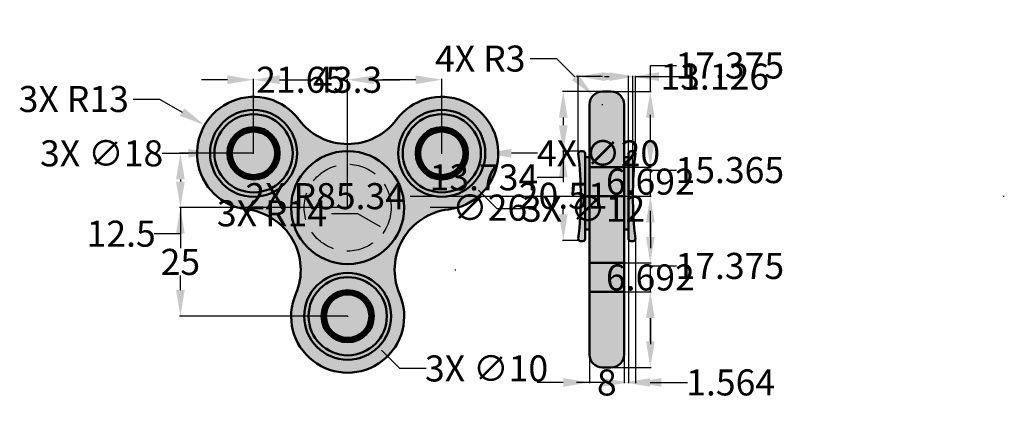
# Model space of a CAD drawing. Units: millimetres. Extents: x 23 to 250, y -22 to 67.
import ezdxf

# ---------------------------------------------------------------- set-up
doc = ezdxf.new("R2010")
doc.units = ezdxf.units.MM
doc.header["$MEASUREMENT"] = 0
doc.linetypes.add('HIDDEN', pattern=[9.525, 6.35, -3.175])
for name, color, linetype, lineweight in [('M-DIMS', 2, 'Continuous', 18), ('M-HATC', 8, 'Continuous', 18), ('M-HIDN', 4, 'HIDDEN', 25), ('M-OUTL', 7, 'Continuous', 50)]:
    doc.layers.add(name, color=color, linetype=linetype, lineweight=lineweight)
doc.styles.get("Standard").update_dxf_attribs({"font": 'arial.ttf'})
doc.dimstyles.get("Standard").update_dxf_attribs({"dimtxt": 6, "dimasz": 6, "dimexe": 0.18, "dimexo": 0.0625, "dimgap": 0.09, "dimtad": 0, "dimtih": 1, "dimtoh": 1, "dimdec": 1, "dimzin": 0, "dimdsep": 46, "dimtxsty": 'Standard', "dimcen": 0.09, "dimadec": 0, "dimazin": 0, "dimtfac": 1, "dimtdec": 1, "dimtofl": 0, "dimtmove": 0, "dimatfit": 3, "dimfxl": 1, "dimtolj": 1, "dimtzin": 0, "dimarcsym": 0})

# ---------------------------------------------------------------- blocks, each defined once
blk = doc.blocks.new('BEARING-SEAT')
for radius in [10, 9, 6, 5]:
    blk.add_circle((10, 10), radius)
blk = doc.blocks.new('FINGER-CAP')
for p, q in [((0.5, 20.69), (1.07, 20.69)), ((0, 10.34), (0, 20.19)), ((0, 10.34), (0, 0.5)), ((0.5, 0), (1.07, 0))]:
    blk.add_line(p, q)
for centre, radius, start, end in [((0.5, 20.19), 0.5, 90, 180), ((1.07, 20.19), 0.5, 353.4148, 90), ((86.34, 10.34), 85.34, 173.4148, 186.5852), ((0.5, 0.5), 0.5, 180, 270), ((1.07, 0.5), 0.5, 270, 6.5852)]:
    blk.add_arc(centre, radius, start, end)
blk = doc.blocks.new('*D3')
at = {"layer": 'Defpoints', "color": 0, "lineweight": 30, "transparency": 16777216}
for p in [(120.56, 53.06), (77.26, 36.13), (120.56, 36.13)]:
    blk.add_point(p, dxfattribs=at)
at = {"layer": 'M-DIMS', "color": 0, "lineweight": -2, "transparency": 16777216}
for p, q in [((77.26, 36.19), (77.26, 53.24)), ((83.26, 53.06), (90.91, 53.06)), ((114.56, 53.06), (106.92, 53.06)), ((120.56, 36.19), (120.56, 53.24))]:
    blk.add_line(p, q, dxfattribs=at)
at = {"layer": 'M-DIMS', "color": 0, "lineweight": 30, "transparency": 16777216}
for points in [[(83.26, 54.06), (83.26, 52.06), (77.26, 53.06)], [(114.56, 54.06), (114.56, 52.06), (120.56, 53.06)]]:
    blk.add_solid(points, dxfattribs=at)
at = {"layer": 'M-DIMS', "color": 0, "transparency": 16777216, "insert": (98.91, 53.06), "char_height": 6, "attachment_point": 5}
blk.add_mtext('\\A1;43.3', dxfattribs=at)
blk = doc.blocks.new('*D4')
at = {"layer": 'Defpoints', "color": 0, "lineweight": 30, "transparency": 16777216}
for p in [(98.91, 53.06), (77.26, 36.13), (98.91, 23.63)]:
    blk.add_point(p, dxfattribs=at)
at = {"layer": 'M-DIMS', "color": 0, "lineweight": -2, "transparency": 16777216}
for p, q in [((71.26, 53.06), (65.26, 53.06)), ((77.26, 36.19), (77.26, 53.24)), ((98.91, 23.69), (98.91, 53.24)), ((104.91, 53.06), (110.91, 53.06))]:
    blk.add_line(p, q, dxfattribs=at)
at = {"layer": 'M-DIMS', "color": 0, "lineweight": 30, "transparency": 16777216}
for points in [[(71.26, 54.06), (71.26, 52.06), (77.26, 53.06)], [(104.91, 54.06), (104.91, 52.06), (98.91, 53.06)]]:
    blk.add_solid(points, dxfattribs=at)
at = {"layer": 'M-DIMS', "color": 0, "transparency": 16777216, "insert": (88.09, 53.06), "char_height": 6, "attachment_point": 5}
blk.add_mtext('\\A1;21.65', dxfattribs=at)
blk = doc.blocks.new('*D5')
at = {"layer": 'Defpoints', "color": 0, "lineweight": 30, "transparency": 16777216}
for p in [(77.26, 36.13), (60.43, 23.63), (98.91, 23.63)]:
    blk.add_point(p, dxfattribs=at)
at = {"layer": 'M-DIMS', "color": 0, "lineweight": -2, "transparency": 16777216}
for p, q in [((77.2, 36.13), (60.25, 36.13)), ((60.43, 30.13), (60.43, 29.63)), ((98.85, 23.63), (60.25, 23.63)), ((60.43, 23.63), (60.43, 17.63)), ((60.43, 17.63), (54.43, 17.63))]:
    blk.add_line(p, q, dxfattribs=at)
at = {"layer": 'M-DIMS', "color": 0, "lineweight": 30, "transparency": 16777216}
for points in [[(59.43, 30.13), (61.43, 30.13), (60.43, 36.13)], [(59.43, 29.63), (61.43, 29.63), (60.43, 23.63)]]:
    blk.add_solid(points, dxfattribs=at)
at = {"layer": 'M-DIMS', "color": 0, "transparency": 16777216, "insert": (46.81, 17.63), "char_height": 6, "attachment_point": 5}
blk.add_mtext('\\A1;12.5', dxfattribs=at)
blk = doc.blocks.new('*D6')
at = {"layer": 'Defpoints', "color": 0, "lineweight": 30, "transparency": 16777216}
for p in [(98.91, 23.63), (60.43, -1.37), (98.91, -1.37)]:
    blk.add_point(p, dxfattribs=at)
at = {"layer": 'M-DIMS', "color": 0, "lineweight": -2, "transparency": 16777216}
for p, q in [((98.85, 23.63), (60.25, 23.63)), ((60.43, 17.63), (60.43, 14.28)), ((60.43, 4.63), (60.43, 7.97)), ((98.85, -1.37), (60.25, -1.37))]:
    blk.add_line(p, q, dxfattribs=at)
at = {"layer": 'M-DIMS', "color": 0, "lineweight": 30, "transparency": 16777216}
for points in [[(59.43, 17.63), (61.43, 17.63), (60.43, 23.63)], [(59.43, 4.63), (61.43, 4.63), (60.43, -1.37)]]:
    blk.add_solid(points, dxfattribs=at)
at = {"layer": 'M-DIMS', "color": 0, "transparency": 16777216, "insert": (60.43, 11.13), "char_height": 6, "attachment_point": 5}
blk.add_mtext('\\A1;25', dxfattribs=at)
blk = doc.blocks.new('*D7')
at = {"layer": 'Defpoints', "color": 0, "lineweight": 30, "transparency": 16777216}
for p in [(154.514575, -10.163581), (162.514575, -10.163581), (162.514575, -16.613581)]:
    blk.add_point(p, dxfattribs=at)
at = {"layer": 'M-DIMS', "color": 0, "lineweight": -2, "transparency": 16777216}
for p, q in [((154.514575, -10.226081), (154.514575, -16.793581)), ((162.514575, -10.226081), (162.514575, -16.793581)), ((148.514575, -16.613581), (142.514575, -16.613581)), ((168.514575, -16.613581), (174.514575, -16.613581))]:
    blk.add_line(p, q, dxfattribs=at)
at = {"layer": 'M-DIMS', "color": 0, "lineweight": 30, "transparency": 16777216}
for points in [[(148.514575, -15.613581), (148.514575, -17.613581), (154.514575, -16.613581)], [(168.514575, -15.613581), (168.514575, -17.613581), (162.514575, -16.613581)]]:
    blk.add_solid(points, dxfattribs=at)
at = {"layer": 'M-DIMS', "color": 0, "transparency": 16777216, "insert": (158.514575, -16.613581), "char_height": 6, "attachment_point": 5}
blk.add_mtext('\\A1;8', dxfattribs=at)
blk = doc.blocks.new('*D8')
at = {"layer": 'Defpoints', "color": 0, "lineweight": 30, "transparency": 16777216}
for p in [(165.08, 53.79), (151.95, 36.06), (165.08, 36.06)]:
    blk.add_point(p, dxfattribs=at)
at = {"layer": 'M-DIMS', "color": 0, "lineweight": -2, "transparency": 16777216}
for p, q in [((151.95, 36.12), (151.95, 53.97)), ((157.95, 53.79), (159.08, 53.79)), ((165.08, 36.12), (165.08, 53.97)), ((165.08, 53.79), (171.08, 53.79))]:
    blk.add_line(p, q, dxfattribs=at)
at = {"layer": 'M-DIMS', "color": 0, "lineweight": 30, "transparency": 16777216}
for points in [[(157.95, 54.79), (157.95, 52.79), (151.95, 53.79)], [(159.08, 54.79), (159.08, 52.79), (165.08, 53.79)]]:
    blk.add_solid(points, dxfattribs=at)
at = {"layer": 'M-DIMS', "color": 0, "transparency": 16777216, "insert": (183.34, 53.79), "char_height": 6, "attachment_point": 5}
blk.add_mtext('\\A1;13.126', dxfattribs=at)
blk = doc.blocks.new('*D9')
at = {"layer": 'Defpoints', "color": 0, "lineweight": 30, "transparency": 16777216}
for p in [(157.51, 50.34), (148.5, 36.6), (152.34, 36.6)]:
    blk.add_point(p, dxfattribs=at)
at = {"layer": 'M-DIMS', "color": 0, "lineweight": -2, "transparency": 16777216}
for p, q in [((157.45, 50.34), (148.32, 50.34)), ((148.5, 44.34), (148.5, 42.6)), ((152.28, 36.6), (148.32, 36.6)), ((148.5, 36.6), (148.5, 30.6)), ((148.5, 30.6), (142.5, 30.6))]:
    blk.add_line(p, q, dxfattribs=at)
at = {"layer": 'M-DIMS', "color": 0, "lineweight": 30, "transparency": 16777216}
for points in [[(147.5, 44.34), (149.5, 44.34), (148.5, 50.34)], [(147.5, 42.6), (149.5, 42.6), (148.5, 36.6)]]:
    blk.add_solid(points, dxfattribs=at)
at = {"layer": 'M-DIMS', "color": 0, "transparency": 16777216, "insert": (130.25, 30.6), "char_height": 6, "attachment_point": 5}
blk.add_mtext('\\A1;13.734', dxfattribs=at)
blk = doc.blocks.new('*D10')
at = {"layer": 'Defpoints', "color": 0, "lineweight": 30, "transparency": 16777216}
for p in [(152.34, 36.6), (148.5, 16.09), (152.07, 16.09)]:
    blk.add_point(p, dxfattribs=at)
at = {"layer": 'M-DIMS', "color": 0, "lineweight": -2, "transparency": 16777216}
for p, q in [((152.28, 36.6), (148.32, 36.6)), ((148.5, 30.6), (148.5, 29.5)), ((148.5, 22.09), (148.5, 23.19)), ((152.01, 16.09), (148.32, 16.09))]:
    blk.add_line(p, q, dxfattribs=at)
at = {"layer": 'M-DIMS', "color": 0, "lineweight": 30, "transparency": 16777216}
for points in [[(147.5, 30.6), (149.5, 30.6), (148.5, 36.6)], [(147.5, 22.09), (149.5, 22.09), (148.5, 16.09)]]:
    blk.add_solid(points, dxfattribs=at)
at = {"layer": 'M-DIMS', "color": 0, "transparency": 16777216, "insert": (148.5, 26.35), "char_height": 6, "attachment_point": 5}
blk.add_mtext('\\A1;20.51', dxfattribs=at)
blk = doc.blocks.new('*D11')
at = {"layer": 'Defpoints', "color": 0, "lineweight": 30, "transparency": 16777216}
for p in [(162.51, 4.21), (168.53, 4.21), (159.51, -13.16)]:
    blk.add_point(p, dxfattribs=at)
at = {"layer": 'M-DIMS', "color": 0, "lineweight": -2, "transparency": 16777216}
for p, q in [((168.53, 4.21), (168.53, 10.21)), ((168.53, 10.21), (174.53, 10.21)), ((162.58, 4.21), (168.71, 4.21)), ((168.53, -7.16), (168.53, -1.79)), ((159.58, -13.16), (168.71, -13.16))]:
    blk.add_line(p, q, dxfattribs=at)
at = {"layer": 'M-DIMS', "color": 0, "lineweight": 30, "transparency": 16777216}
for points in [[(167.53, -1.79), (169.53, -1.79), (168.53, 4.21)], [(167.53, -7.16), (169.53, -7.16), (168.53, -13.16)]]:
    blk.add_solid(points, dxfattribs=at)
at = {"layer": 'M-DIMS', "color": 0, "transparency": 16777216, "insert": (186.81, 10.21), "char_height": 6, "attachment_point": 5}
blk.add_mtext('\\A1;17.375', dxfattribs=at)
blk = doc.blocks.new('*D12')
at = {"layer": 'Defpoints', "color": 0, "lineweight": 30, "transparency": 16777216}
for p in [(162.514575, 10.903671), (168.528589, 10.903671), (162.514575, 4.211419)]:
    blk.add_point(p, dxfattribs=at)
at = {"layer": 'M-DIMS', "color": 0, "lineweight": -2, "transparency": 16777216}
for p, q in [((168.528589, 16.903671), (168.528589, 22.903671)), ((162.577075, 10.903671), (168.708589, 10.903671)), ((162.577075, 4.211419), (168.708589, 4.211419)), ((168.528589, -1.788581), (168.528589, -7.788581))]:
    blk.add_line(p, q, dxfattribs=at)
at = {"layer": 'M-DIMS', "color": 0, "lineweight": 30, "transparency": 16777216}
for points in [[(167.528589, 16.903671), (169.528589, 16.903671), (168.528589, 10.903671)], [(167.528589, -1.788581), (169.528589, -1.788581), (168.528589, 4.211419)]]:
    blk.add_solid(points, dxfattribs=at)
at = {"layer": 'M-DIMS', "color": 0, "transparency": 16777216, "insert": (168.528589, 7.557545), "char_height": 6, "attachment_point": 5}
blk.add_mtext('\\A1;6.692', dxfattribs=at)
blk = doc.blocks.new('*D13')
at = {"layer": 'Defpoints', "color": 0, "lineweight": 30, "transparency": 16777216}
for p in [(162.51, 26.27), (168.53, 26.27), (162.51, 10.9)]:
    blk.add_point(p, dxfattribs=at)
at = {"layer": 'M-DIMS', "color": 0, "lineweight": -2, "transparency": 16777216}
for p, q in [((168.53, 26.27), (168.53, 32.27)), ((168.53, 32.27), (174.53, 32.27)), ((162.58, 26.27), (168.71, 26.27)), ((168.53, 16.9), (168.53, 20.27)), ((162.58, 10.9), (168.71, 10.9))]:
    blk.add_line(p, q, dxfattribs=at)
at = {"layer": 'M-DIMS', "color": 0, "lineweight": 30, "transparency": 16777216}
for points in [[(167.53, 20.27), (169.53, 20.27), (168.53, 26.27)], [(167.53, 16.9), (169.53, 16.9), (168.53, 10.9)]]:
    blk.add_solid(points, dxfattribs=at)
at = {"layer": 'M-DIMS', "color": 0, "transparency": 16777216, "insert": (186.81, 32.27), "char_height": 6, "attachment_point": 5}
blk.add_mtext('\\A1;15.365', dxfattribs=at)
blk = doc.blocks.new('*D14')
at = {"layer": 'Defpoints', "color": 0, "lineweight": 30, "transparency": 16777216}
for p in [(162.514575, 32.961419), (168.528589, 32.961419), (162.514575, 26.269167)]:
    blk.add_point(p, dxfattribs=at)
at = {"layer": 'M-DIMS', "color": 0, "lineweight": -2, "transparency": 16777216}
for p, q in [((168.528589, 38.961419), (168.528589, 44.961419)), ((162.577075, 32.961419), (168.708589, 32.961419)), ((162.577075, 26.269167), (168.708589, 26.269167)), ((168.528589, 20.269167), (168.528589, 14.269167))]:
    blk.add_line(p, q, dxfattribs=at)
at = {"layer": 'M-DIMS', "color": 0, "lineweight": 30, "transparency": 16777216}
for points in [[(167.528589, 38.961419), (169.528589, 38.961419), (168.528589, 32.961419)], [(167.528589, 20.269167), (169.528589, 20.269167), (168.528589, 26.269167)]]:
    blk.add_solid(points, dxfattribs=at)
at = {"layer": 'M-DIMS', "color": 0, "transparency": 16777216, "insert": (168.528589, 29.615293), "char_height": 6, "attachment_point": 5}
blk.add_mtext('\\A1;6.692', dxfattribs=at)
blk = doc.blocks.new('*D15')
at = {"layer": 'Defpoints', "color": 0, "lineweight": 30, "transparency": 16777216}
for p in [(159.51, 50.34), (168.53, 50.34), (162.51, 32.96)]:
    blk.add_point(p, dxfattribs=at)
at = {"layer": 'M-DIMS', "color": 0, "lineweight": -2, "transparency": 16777216}
for p, q in [((168.53, 50.34), (168.53, 56.34)), ((168.53, 56.34), (174.53, 56.34)), ((159.58, 50.34), (168.71, 50.34)), ((168.53, 38.96), (168.53, 44.34)), ((162.58, 32.96), (168.71, 32.96))]:
    blk.add_line(p, q, dxfattribs=at)
at = {"layer": 'M-DIMS', "color": 0, "lineweight": 30, "transparency": 16777216}
for points in [[(167.53, 44.34), (169.53, 44.34), (168.53, 50.34)], [(167.53, 38.96), (169.53, 38.96), (168.53, 32.96)]]:
    blk.add_solid(points, dxfattribs=at)
at = {"layer": 'M-DIMS', "color": 0, "transparency": 16777216, "insert": (186.81, 56.34), "char_height": 6, "attachment_point": 5}
blk.add_mtext('\\A1;17.375', dxfattribs=at)
blk = doc.blocks.new('*D16')
at = {"layer": 'Defpoints', "color": 0, "lineweight": 30, "transparency": 16777216}
for p in [(163.51, 16.42), (165.08, 16.38), (165.08, -16.61)]:
    blk.add_point(p, dxfattribs=at)
at = {"layer": 'M-DIMS', "color": 0, "lineweight": -2, "transparency": 16777216}
for p, q in [((163.51, 16.36), (163.51, -16.79)), ((165.08, 16.31), (165.08, -16.79)), ((157.51, -16.61), (151.51, -16.61)), ((171.08, -16.61), (177.08, -16.61))]:
    blk.add_line(p, q, dxfattribs=at)
at = {"layer": 'M-DIMS', "color": 0, "lineweight": 30, "transparency": 16777216}
for points in [[(157.51, -15.61), (157.51, -17.61), (163.51, -16.61)], [(171.08, -15.61), (171.08, -17.61), (165.08, -16.61)]]:
    blk.add_solid(points, dxfattribs=at)
at = {"layer": 'M-DIMS', "color": 0, "transparency": 16777216, "insert": (187, -16.61), "char_height": 6, "attachment_point": 5}
blk.add_mtext('\\A1;1.564', dxfattribs=at)
blk = doc.blocks.new('*D17')
at = {"layer": 'Defpoints', "color": 0, "lineweight": 30, "transparency": 16777216}
for p in [(164.51, 53.79), (163.51, 26.27), (164.51, 26.27)]:
    blk.add_point(p, dxfattribs=at)
at = {"layer": 'M-DIMS', "color": 0, "lineweight": -2, "transparency": 16777216}
for p, q in [((157.51, 53.79), (151.51, 53.79)), ((163.51, 26.33), (163.51, 53.97)), ((164.51, 26.33), (164.51, 53.97)), ((170.51, 53.79), (176.51, 53.79))]:
    blk.add_line(p, q, dxfattribs=at)
at = {"layer": 'M-DIMS', "color": 0, "lineweight": 30, "transparency": 16777216}
for points in [[(157.51, 54.79), (157.51, 52.79), (163.51, 53.79)], [(170.51, 54.79), (170.51, 52.79), (164.51, 53.79)]]:
    blk.add_solid(points, dxfattribs=at)
at = {"layer": 'M-DIMS', "color": 0, "transparency": 16777216, "insert": (177.71, 53.79), "char_height": 6, "attachment_point": 5}
blk.add_mtext('\\A1;1', dxfattribs=at)
blk = doc.blocks.new('*D18')
at = {"layer": 'Defpoints', "color": 0, "lineweight": 30, "transparency": 16777216}
for p in [(85.91, 23.63), (111.91, 23.63)]:
    blk.add_point(p, dxfattribs=at)
at = {"layer": 'M-DIMS', "color": 0, "lineweight": -2, "transparency": 16777216}
for p, q in [((98.82, 23.63), (99, 23.63)), ((98.91, 23.54), (98.91, 23.72)), ((123.91, 23.63), (117.91, 23.63))]:
    blk.add_line(p, q, dxfattribs=at)
at = {"layer": 'M-DIMS', "color": 0, "lineweight": 30, "transparency": 16777216}
blk.add_solid([(117.91, 24.63), (117.91, 22.63), (111.91, 23.63)], dxfattribs=at)
at = {"layer": 'M-DIMS', "color": 0, "transparency": 16777216, "insert": (131.56, 23.63), "char_height": 6, "attachment_point": 5}
blk.add_mtext('\\A1;∅26', dxfattribs=at)
blk = doc.blocks.new('*D19')
at = {"layer": 'Defpoints', "color": 0, "lineweight": 30, "transparency": 16777216}
for p in [(110.56, 36.13), (130.56, 36.13)]:
    blk.add_point(p, dxfattribs=at)
at = {"layer": 'M-DIMS', "color": 0, "lineweight": -2, "transparency": 16777216}
for p, q in [((120.47, 36.13), (120.65, 36.13)), ((120.56, 36.04), (120.56, 36.22)), ((142.56, 36.13), (136.56, 36.13))]:
    blk.add_line(p, q, dxfattribs=at)
at = {"layer": 'M-DIMS', "color": 0, "lineweight": 30, "transparency": 16777216}
blk.add_solid([(136.56, 37.13), (136.56, 35.13), (130.56, 36.13)], dxfattribs=at)
at = {"layer": 'M-DIMS', "color": 0, "transparency": 16777216, "insert": (156.61, 36.13), "char_height": 6, "attachment_point": 5}
blk.add_mtext('\\A1;4X ∅20', dxfattribs=at)
blk = doc.blocks.new('*D20')
at = {"layer": 'Defpoints', "color": 0, "lineweight": 30, "transparency": 16777216}
for p in [(68.26, 36.13), (86.26, 36.13)]:
    blk.add_point(p, dxfattribs=at)
at = {"layer": 'M-DIMS', "color": 0, "lineweight": -2, "transparency": 16777216}
for p, q in [((56.26, 36.13), (62.26, 36.13)), ((77.17, 36.13), (77.35, 36.13)), ((77.26, 36.04), (77.26, 36.22))]:
    blk.add_line(p, q, dxfattribs=at)
at = {"layer": 'M-DIMS', "color": 0, "lineweight": 30, "transparency": 16777216}
blk.add_solid([(62.26, 37.13), (62.26, 35.13), (68.26, 36.13)], dxfattribs=at)
at = {"layer": 'M-DIMS', "color": 0, "transparency": 16777216, "insert": (42.32, 36.13), "char_height": 6, "attachment_point": 5}
blk.add_mtext('\\A1;3X ∅18', dxfattribs=at)
blk = doc.blocks.new('*D21')
at = {"layer": 'Defpoints', "color": 0, "lineweight": 30, "transparency": 16777216}
for p in [(116.33, 40.37), (124.8, 31.88)]:
    blk.add_point(p, dxfattribs=at)
at = {"layer": 'M-DIMS', "color": 0, "lineweight": -2, "transparency": 16777216}
for p, q in [((120.47, 36.13), (120.65, 36.13)), ((120.56, 36.04), (120.56, 36.22)), ((133.28, 23.38), (129.04, 27.63)), ((139.28, 23.38), (133.28, 23.38))]:
    blk.add_line(p, q, dxfattribs=at)
at = {"layer": 'M-DIMS', "color": 0, "lineweight": 30, "transparency": 16777216}
blk.add_solid([(129.75, 28.34), (128.33, 26.93), (124.8, 31.88)], dxfattribs=at)
at = {"layer": 'M-DIMS', "color": 0, "transparency": 16777216, "insert": (153.18, 23.38), "char_height": 6, "attachment_point": 5}
blk.add_mtext('\\A1;3X ∅12', dxfattribs=at)
blk = doc.blocks.new('*D22')
at = {"layer": 'Defpoints', "color": 0, "lineweight": 30, "transparency": 16777216}
for p in [(95.38, 2.16), (102.45, -4.91)]:
    blk.add_point(p, dxfattribs=at)
at = {"layer": 'M-DIMS', "color": 0, "lineweight": -2, "transparency": 16777216}
for p, q in [((98.82, -1.37), (99, -1.37)), ((98.91, -1.46), (98.91, -1.28)), ((110.93, -13.39), (106.69, -9.15)), ((116.93, -13.39), (110.93, -13.39))]:
    blk.add_line(p, q, dxfattribs=at)
at = {"layer": 'M-DIMS', "color": 0, "lineweight": 30, "transparency": 16777216}
blk.add_solid([(107.4, -8.44), (105.98, -9.86), (102.45, -4.91)], dxfattribs=at)
at = {"layer": 'M-DIMS', "color": 0, "transparency": 16777216, "insert": (130.86, -13.39), "char_height": 6, "attachment_point": 5}
blk.add_mtext('\\A1;3X ∅10', dxfattribs=at)
blk = doc.blocks.new('*D23')
at = {"layer": 'Defpoints', "color": 0, "lineweight": 30, "transparency": 16777216}
for p in [(66, 42.63), (77.26, 36.13)]:
    blk.add_point(p, dxfattribs=at)
at = {"layer": 'M-DIMS', "color": 0, "lineweight": -2, "transparency": 16777216}
for p, q in [((49.61, 48.63), (55.61, 48.63)), ((55.61, 48.63), (60.81, 45.63)), ((77.17, 36.13), (77.35, 36.13)), ((77.26, 36.04), (77.26, 36.22))]:
    blk.add_line(p, q, dxfattribs=at)
at = {"layer": 'M-DIMS', "color": 0, "lineweight": 30, "transparency": 16777216}
blk.add_solid([(61.31, 46.49), (60.31, 44.76), (66, 42.63)], dxfattribs=at)
at = {"layer": 'M-DIMS', "color": 0, "transparency": 16777216, "insert": (35.91, 48.63), "char_height": 6, "attachment_point": 5}
blk.add_mtext('\\A1;3X R13', dxfattribs=at)
blk = doc.blocks.new('*D24')
at = {"layer": 'Defpoints', "color": 0, "lineweight": 30, "transparency": 16777216}
for p in [(111.58, 16.31), (123.71, 9.31)]:
    blk.add_point(p, dxfattribs=at)
at = {"layer": 'M-DIMS', "color": 0, "lineweight": -2, "transparency": 16777216}
for p, q in [((95.19, 22.31), (101.19, 22.31)), ((101.19, 22.31), (106.39, 19.31)), ((123.62, 9.31), (123.8, 9.31)), ((123.71, 9.22), (123.71, 9.4))]:
    blk.add_line(p, q, dxfattribs=at)
at = {"layer": 'M-DIMS', "color": 0, "lineweight": 30, "transparency": 16777216}
blk.add_solid([(106.89, 20.18), (105.89, 18.45), (111.58, 16.31)], dxfattribs=at)
at = {"layer": 'M-DIMS', "color": 0, "transparency": 16777216, "insert": (81.5, 22.31), "char_height": 6, "attachment_point": 5}
blk.add_mtext('\\A1;3X R14', dxfattribs=at)
blk = doc.blocks.new('*D25')
at = {"layer": 'Defpoints', "color": 0, "lineweight": 30, "transparency": 16777216}
for p in [(164.51, 26.27), (249.86, 26.27)]:
    blk.add_point(p, dxfattribs=at)
at = {"layer": 'M-DIMS', "color": 0, "lineweight": -2, "transparency": 16777216}
for p, q in [((113.31, 26.27), (158.51, 26.27)), ((249.77, 26.27), (249.95, 26.27)), ((249.86, 26.18), (249.86, 26.36))]:
    blk.add_line(p, q, dxfattribs=at)
at = {"layer": 'M-DIMS', "color": 0, "lineweight": 30, "transparency": 16777216}
blk.add_solid([(158.51, 27.27), (158.51, 25.27), (164.51, 26.27)], dxfattribs=at)
at = {"layer": 'M-DIMS', "color": 0, "transparency": 16777216, "insert": (93.74, 26.27), "char_height": 6, "attachment_point": 5}
blk.add_mtext('\\A1;2X R85.34', dxfattribs=at)
blk = doc.blocks.new('*D26')
at = {"layer": 'Defpoints', "color": 0, "lineweight": 30, "transparency": 16777216}
for p in [(155.39, 49.46), (157.51, 47.34)]:
    blk.add_point(p, dxfattribs=at)
at = {"layer": 'M-DIMS', "color": 0, "lineweight": -2, "transparency": 16777216}
for p, q in [((140.91, 57.94), (146.91, 57.94)), ((146.91, 57.94), (151.15, 53.7)), ((157.42, 47.34), (157.6, 47.34)), ((157.51, 47.25), (157.51, 47.43))]:
    blk.add_line(p, q, dxfattribs=at)
at = {"layer": 'M-DIMS', "color": 0, "lineweight": 30, "transparency": 16777216}
blk.add_solid([(151.86, 54.41), (150.44, 52.99), (155.39, 49.46)], dxfattribs=at)
at = {"layer": 'M-DIMS', "color": 0, "transparency": 16777216, "insert": (129.41, 57.94), "char_height": 6, "attachment_point": 5}
blk.add_mtext('\\A1;4X R3', dxfattribs=at)

msp = doc.modelspace()

# ---------------------------------------------------------------- hatches: boundary and pattern name
at = {"layer": 'M-HATC'}
h = msp.add_hatch(color=256, dxfattribs=at)
h.dxf.hatch_style = 1
h.set_gradient(color1=(237, 31, 36), color2=(248, 153, 30), tint=1)
h.paths.add_polyline_path([(162.5146, 47.3364, 0.41421356), (159.5146, 50.3364), (157.5146, 50.3364, 0.41421356), (154.5146, 47.3364), (154.5146, 32.9614), (162.5146, 32.9614), (162.5146, 35.2241)])
h.paths.add_polyline_path([(162.5146, 26.2692), (154.5146, 26.2692), (154.5146, 10.9037), (162.5146, 10.9037)])
h.paths.add_polyline_path([(162.5146, 4.2114), (154.5146, 4.2114), (154.5146, -10.1636, 0.41421356), (157.5146, -13.1636), (159.5146, -13.1636, 0.41421356), (162.5146, -10.1636)])
h = msp.add_hatch(color=256, dxfattribs=at)
h.dxf.hatch_style = 1
h.set_gradient(color1=(205, 32, 39), color2=(255, 255, 0), tint=1)
h.paths.add_polyline_path([(110.139, 43.8941, -0.50195914), (87.6865, 43.8941, 1.51973937), (75.7475, 23.2152, -0.50195914), (86.9738, 3.7708, 1.51973937), (110.8517, 3.7708, -0.50195914), (122.0779, 23.2152, 1.51973937)])
h.paths.add_polyline_path([(111.9127, 23.6267, -1), (85.9127, 23.6267, -1)], flags=16)
h.paths.add_polyline_path([(67.2621, 36.1267, -1), (87.2621, 36.1267, -1)], flags=16)
h.paths.add_polyline_path([(108.9127, 23.6267, -1), (88.9127, 23.6267, -1)], flags=0)
h.paths.add_polyline_path([(68.2621, 36.1267, -1), (86.2621, 36.1267, -1)], flags=0)
h.paths.add_polyline_path([(71.2621, 36.1267, -1), (83.2621, 36.1267, -1)], flags=0)
h.paths.add_polyline_path([(72.2621, 36.1267, -1), (82.2621, 36.1267, -1)], flags=0)
h.paths.add_polyline_path([(108.9127, -1.3733, -1), (88.9127, -1.3733, -1)], flags=16)
h.paths.add_polyline_path([(107.9127, -1.3733, -1), (89.9127, -1.3733, -1)], flags=0)
h.paths.add_polyline_path([(104.9127, -1.3733, -1), (92.9127, -1.3733, -1)], flags=0)
h.paths.add_polyline_path([(103.9127, -1.3733, -1), (93.9127, -1.3733, -1)], flags=0)
h.paths.add_polyline_path([(110.5633, 36.1267, -1), (130.5633, 36.1267, -1)], flags=16)
h.paths.add_polyline_path([(111.5633, 36.1267, -1), (129.5633, 36.1267, -1)], flags=0)
h.paths.add_polyline_path([(114.5633, 36.1267, -1), (126.5633, 36.1267, -1)], flags=0)
h.paths.add_polyline_path([(115.5633, 36.1267, -1), (125.5633, 36.1267, -1)], flags=0)
h = msp.add_hatch(color=256, dxfattribs=at)
h.dxf.hatch_style = 1
h.set_gradient(color1=(69, 84, 165), color2=(237, 31, 36), tint=1)
h.paths.add_polyline_path([(67.2621, 36.1267, 1), (87.2621, 36.1267, 1)])
h.paths.add_polyline_path([(86.2621, 36.1267, -1), (68.2621, 36.1267, -1)], flags=16)
h.paths.add_polyline_path([(83.2621, 36.1267, -1), (71.2621, 36.1267, -1)], flags=0)
h.paths.add_polyline_path([(82.2621, 36.1267, -1), (72.2621, 36.1267, -1)], flags=0)
h.paths.add_polyline_path([(111.9127, 23.6267, 1), (85.9127, 23.6267, 1)])
h.paths.add_polyline_path([(88.9127, 23.6267, -1), (108.9127, 23.6267, -1)], flags=16)
h.paths.add_polyline_path([(110.5633, 36.1267, 1), (130.5633, 36.1267, 1)])
h.paths.add_polyline_path([(129.5633, 36.1267, -1), (111.5633, 36.1267, -1)], flags=16)
h.paths.add_polyline_path([(126.5633, 36.1267, -1), (114.5633, 36.1267, -1)], flags=0)
h.paths.add_polyline_path([(125.5633, 36.1267, -1), (115.5633, 36.1267, -1)], flags=0)
h.paths.add_polyline_path([(88.9127, -1.3733, 1), (108.9127, -1.3733, 1)])
h.paths.add_polyline_path([(107.9127, -1.3733, -1), (89.9127, -1.3733, -1)], flags=16)
h.paths.add_polyline_path([(104.9127, -1.3733, -1), (92.9127, -1.3733, -1)], flags=0)
h.paths.add_polyline_path([(103.9127, -1.3733, -1), (93.9127, -1.3733, -1)], flags=0)
h = msp.add_hatch(color=256, dxfattribs=at)
h.dxf.hatch_style = 1
h.set_gradient(color1=(205, 32, 39), color2=(255, 255, 0), tint=1)
h.paths.add_polyline_path([(86.2621, 36.1267, 1), (68.2621, 36.1267, 1)])
h.paths.add_polyline_path([(71.2621, 36.1267, -1), (83.2621, 36.1267, -1)], flags=16)
h.paths.add_polyline_path([(72.2621, 36.1267, -1), (82.2621, 36.1267, -1)], flags=0)
h.paths.add_polyline_path([(129.5633, 36.1267, 1), (111.5633, 36.1267, 1)])
h.paths.add_polyline_path([(114.5633, 36.1267, -1), (126.5633, 36.1267, -1)], flags=16)
h.paths.add_polyline_path([(115.5633, 36.1267, -1), (125.5633, 36.1267, -1)], flags=0)
h.paths.add_polyline_path([(89.9127, -1.3733, 1), (107.9127, -1.3733, 1)])
h.paths.add_polyline_path([(104.9127, -1.3733, -1), (92.9127, -1.3733, -1)], flags=16)
h.paths.add_polyline_path([(103.9127, -1.3733, -1), (93.9127, -1.3733, -1)], flags=0)
h = msp.add_hatch(dxfattribs=at)
h.set_pattern_fill('ANSI31', color=256)
h.paths.add_polyline_path([(71.2621, 36.1267, 1), (83.2621, 36.1267, 1)])
h.paths.add_polyline_path([(82.2621, 36.1267, -1), (72.2621, 36.1267, -1)], flags=16)
h.paths.add_polyline_path([(114.5633, 36.1267, 1), (126.5633, 36.1267, 1)])
h.paths.add_polyline_path([(125.5633, 36.1267, -1), (115.5633, 36.1267, -1)], flags=16)
h.paths.add_polyline_path([(104.9127, -1.3733, 1), (92.9127, -1.3733, 1)])
h.paths.add_polyline_path([(93.9127, -1.3733, -1), (103.9127, -1.3733, -1)], flags=16)
h = msp.add_hatch(color=256, dxfattribs=at)
h.dxf.hatch_style = 1
h.set_gradient(color1=(205, 105, 40), color2=(237, 31, 36), tint=1)
h.paths.add_polyline_path([(88.9127, 23.6267, 1), (108.9127, 23.6267, 1)])
h.paths.add_polyline_path([(125.5633, 36.1267, 1), (115.5633, 36.1267, 1)])
h.paths.add_polyline_path([(103.9127, -1.3733, 1), (93.9127, -1.3733, 1)])
h.paths.add_polyline_path([(82.2621, 36.1267, 1), (72.2621, 36.1267, 1)])
h = msp.add_hatch(color=256, dxfattribs=at)
h.dxf.hatch_style = 1
h.set_gradient(color1=(153, 27, 30), color2=(248, 246, 176))
h.paths.add_polyline_path([(153.5146, 36.1137, 0.41421356), (153.0146, 36.6137), (152.4482, 36.6137, 0.44829183), (151.9515, 36.0564, -0.05753018), (151.9515, 16.482, 0.44829183), (152.4482, 15.9246), (153.0146, 15.9246, 0.41421356), (153.5146, 16.4246), (153.5146, 26.2692)])
h = msp.add_hatch(color=256, dxfattribs=at)
h.dxf.hatch_style = 1
h.set_gradient(color1=(153, 27, 30), color2=(248, 246, 176))
h.paths.add_polyline_path([(165.0776, 36.0564, 0.44829183), (164.5809, 36.6137), (164.0146, 36.6137, 0.41421356), (163.5146, 36.1137), (163.5146, 26.2692), (163.5146, 16.4246, 0.41421356), (164.0146, 15.9246), (164.5809, 15.9246, 0.44829183), (165.0776, 16.482, -0.05753018)])
h = msp.add_hatch(color=256, dxfattribs=at)
h.dxf.hatch_style = 1
h.set_gradient(color1=(153, 27, 30), color2=(248, 246, 176))
h.paths.add_polyline_path([(154.5146, 35.2241), (153.5146, 35.2241), (153.5146, 26.2692), (153.5146, 18.5864), (154.5146, 18.5864)])
h = msp.add_hatch(color=256, dxfattribs=at)
h.dxf.hatch_style = 1
h.set_gradient(color1=(153, 27, 30), color2=(248, 246, 176))
h.paths.add_polyline_path([(163.5146, 35.2241), (162.5146, 35.2241), (162.5146, 26.2692), (162.5146, 18.5864), (163.5146, 18.5864), (163.5146, 26.2692)])
h = msp.add_hatch(color=256, dxfattribs=at)
h.dxf.hatch_style = 1
h.set_gradient(color1=(39, 118, 187), color2=(242, 103, 34), tint=1)
h.paths.add_polyline_path([(162.5146, 32.9614), (154.5146, 32.9614), (154.5146, 26.2692), (162.5146, 26.2692)])
h.paths.add_polyline_path([(162.5146, 10.9037), (154.5146, 10.9037), (154.5146, 4.2114), (162.5146, 4.2114)])

# ---------------------------------------------------------------- linework, layer by layer
at = {"layer": 'M-HIDN'}
msp.add_circle((98.9127, 23.6267), 10, dxfattribs=at)
at = {"layer": 'M-OUTL'}
for p, q in [((157.5146, 50.3364), (159.5146, 50.3364)), ((154.5146, -10.1636), (154.5146, 47.3364)), ((162.5146, 47.3364), (162.5146, -10.1636)), ((162.5146, 47.3364), (162.5146, 18.5864)), ((154.5146, 35.2241), (153.5146, 35.2241)), ((162.5146, 26.2692), (162.5146, 35.2241)), ((162.5146, 35.2241), (163.5146, 35.2241)), ((162.5146, 32.9614), (154.5146, 32.9614)), ((162.5146, 32.9614), (162.5146, 14.1706)), ((162.5146, 26.2692), (154.5146, 26.2692)), ((162.5146, 26.2692), (162.5146, 17.3143)), ((154.5146, 18.5864), (153.5146, 18.5864)), ((162.5146, 18.5864), (163.5146, 18.5864)), ((162.5146, 10.9037), (154.5146, 10.9037)), ((162.5146, 4.2114), (154.5146, 4.2114)), ((157.5146, -13.1636), (159.5146, -13.1636)), ((159.5146, -13.1636), (157.5146, -13.1636))]:
    msp.add_line(p, q, dxfattribs=at)
msp.add_circle((98.9127, 23.6267), 13, dxfattribs=at)
for centre, radius, start, end in [((157.5146, 47.3364), 3, 90, 180), ((159.5146, 47.3364), 3, 0, 90), ((77.2621, 36.1267), 13, 36.690438, 263.309562), ((120.5633, 36.1267), 13, 276.690438, 143.309562), ((98.9127, 52.2589), 14, 216.690438, 323.309562), ((74.1164, 9.3105), 14, 336.690438, 83.309562), ((123.709, 9.3105), 14, 96.690438, 203.309562), ((98.9127, -1.3733), 13, 156.690438, 23.309562), ((157.5146, -10.1636), 3, 180, 270), ((159.5146, -10.1636), 3, 270, 0)]:
    msp.add_arc(centre, radius, start, end, dxfattribs=at)

# ---------------------------------------------------------------- block references
for name, p, rotation in [('BEARING-SEAT', (87.2621, 26.1267), 90), ('BEARING-SEAT', (130.5633, 26.1267), 90), ('FINGER-CAP', (153.5142, 36.6133), 180)]:
    msp.add_blockref(name, p, dxfattribs=dict(at, rotation=rotation))
for name, p in [('FINGER-CAP', (163.515, 15.925)), ('BEARING-SEAT', (88.9127, -11.3733))]:
    msp.add_blockref(name, p, dxfattribs=at)

# ---------------------------------------------------------------- dimensions: what is measured, and where the dimension line sits
at = {"layer": 'M-DIMS'}
for center, mpoint, text, picture, middle in [((157.5146, 47.3364), (155.3933, 49.4577), '4X <>', '*D26', (129.4135, 57.943)), ((77.2621, 36.1267), (66.004, 42.627), '3X <>', '*D23', (35.9093, 48.6274)), ((123.709, 9.3105), (111.5849, 16.311), '3X <>', '*D24', (81.5026, 22.3115))]:
    dim = msp.add_radius_dim(center=center, mpoint=mpoint, text=text, dimstyle='Standard', override={"dimdec": 0, "dimlfac": 1, "dimrnd": 0, "dimzin": 0, "dimdsep": 46, "dimlunit": 2}, dxfattribs=at)
    dim.commit()
    dim.dimension.update_dxf_attribs({"geometry": picture, "text_midpoint": middle})
for base, p1, p2, override, picture, middle in [((168.5286, 50.3364), (162.5146, 32.9614), (159.5146, 50.3364), {"dimdec": 3, "dimlfac": 1, "dimrnd": 0, "dimzin": 0, "dimdsep": 46, "dimlunit": 2}, '*D15', (186.813, 56.3364)), ((148.5006, 36.6025), (157.5146, 50.3364), (152.3431, 36.6025), {"dimdec": 3, "dimlfac": 1, "dimrnd": 0, "dimzin": 0, "dimdsep": 46, "dimlunit": 2}, '*D9', (130.2509, 30.6025)), ((168.5286, 32.9614), (162.5146, 26.2692), (162.5146, 32.9614), {"dimdec": 3, "dimlfac": 1, "dimrnd": 0, "dimzin": 0, "dimdsep": 46, "dimlunit": 2}, '*D14', (168.5286, 29.6153)), ((148.5006, 16.092), (152.3431, 36.6025), (152.0749, 16.092), {"dimdec": 2, "dimlfac": 1, "dimrnd": 0, "dimzin": 0, "dimdsep": 46, "dimlunit": 2}, '*D10', (148.5006, 26.3472)), ((60.4314, 23.6267), (77.2621, 36.1267), (98.9127, 23.6267), {"dimdec": 1, "dimlfac": 1, "dimrnd": 0, "dimzin": 0, "dimdsep": 46, "dimlunit": 2}, '*D5', (46.8087, 17.6267)), ((168.528589, 26.269167), (162.514575, 10.903671), (162.514575, 26.269167), {"dimdec": 3, "dimlfac": 1, "dimrnd": 0, "dimzin": 0, "dimdsep": 46, "dimlunit": 2}, '*D13', (186.812996, 32.269167)), ((60.4314, -1.3733), (98.9127, 23.6267), (98.9127, -1.3733), {"dimdec": 0, "dimlfac": 1, "dimrnd": 0, "dimzin": 0, "dimdsep": 46, "dimlunit": 2}, '*D6', (60.4314, 11.1267)), ((168.5286, 10.9037), (162.5146, 4.2114), (162.5146, 10.9037), {"dimdec": 3, "dimlfac": 1, "dimrnd": 0, "dimzin": 0, "dimdsep": 46, "dimlunit": 2}, '*D12', (168.5286, 7.5575)), ((168.5286, 4.2114), (159.5146, -13.1636), (162.5146, 4.2114), {"dimdec": 3, "dimlfac": 1, "dimrnd": 0, "dimzin": 0, "dimdsep": 46, "dimlunit": 2}, '*D11', (186.813, 10.2114))]:
    dim = msp.add_linear_dim(base=base, p1=p1, p2=p2, angle=90, dimstyle='Standard', override=override, dxfattribs=at)
    dim.commit()
    dim.dimension.update_dxf_attribs({"geometry": picture, "text_midpoint": middle})
for base, p1, p2, override, picture, middle in [((98.9127, 53.0588), (77.2621, 36.1267), (98.9127, 23.6267), {"dimdec": 2, "dimlfac": 1, "dimrnd": 0, "dimzin": 0, "dimdsep": 46, "dimlunit": 2}, '*D4', (88.0874, 53.0588)), ((120.5633, 53.0588), (77.2621, 36.1267), (120.5633, 36.1267), {"dimdec": 1, "dimlfac": 1, "dimrnd": 0, "dimzin": 0, "dimdsep": 46, "dimlunit": 2}, '*D3', (98.9127, 53.0588)), ((164.5146, 53.7864), (163.5146, 26.2692), (164.5146, 26.2692), {"dimdec": 0, "dimlfac": 1, "dimrnd": 0, "dimzin": 0, "dimdsep": 46, "dimlunit": 2}, '*D17', (177.7096, 53.7864)), ((165.0776, 53.7864), (151.9515, 36.0564), (165.0776, 36.0564), {"dimdec": 3, "dimlfac": 1, "dimrnd": 0, "dimzin": 0, "dimdsep": 46, "dimlunit": 2}, '*D8', (183.3375, 53.7864)), ((165.0786, -16.6136), (163.5146, 16.4246), (165.0786, 16.3762), {"dimdec": 3, "dimlfac": 1, "dimrnd": 0, "dimzin": 0, "dimdsep": 46, "dimlunit": 2}, '*D16', (186.9974, -16.6136)), ((162.5146, -16.6136), (154.5146, -10.1636), (162.5146, -10.1636), {"dimdec": 0, "dimlfac": 1, "dimrnd": 0, "dimzin": 0, "dimdsep": 46, "dimlunit": 2}, '*D7', (158.5146, -16.6136))]:
    dim = msp.add_linear_dim(base=base, p1=p1, p2=p2, dimstyle='Standard', override=override, dxfattribs=at)
    dim.commit()
    dim.dimension.update_dxf_attribs({"geometry": picture, "text_midpoint": middle})
for p1, p2, text, picture, middle in [((86.2621, 36.1263), (68.2621, 36.127), '3X <>', '*D20', (56.2621, 36.1274)), ((110.5633, 36.1263), (130.5633, 36.127), '4X <>', '*D19', (142.5633, 36.1274)), ((116.3257, 40.3743), (124.801, 31.879), '3X <>', '*D21', (153.1814, 23.3837)), ((95.3769, 2.1619), (102.4486, -4.9086), '3X <>', '*D22', (130.8602, -13.3931))]:
    dim = msp.add_diameter_dim_2p(p1=p1, p2=p2, text=text, dimstyle='Standard', override={"dimdec": 0, "dimlfac": 1, "dimrnd": 0, "dimzin": 0, "dimdsep": 46, "dimlunit": 2}, dxfattribs=at)
    dim.commit()
    dim.dimension.update_dxf_attribs({"geometry": picture, "text_midpoint": middle, "dimtype": 163})
dim = msp.add_radius_dim(center=(249.8575, 26.2692), mpoint=(164.5146, 26.269), text='2X <>', dimstyle='Standard', override={"dimdec": 2, "dimlfac": 1, "dimrnd": 0, "dimzin": 0, "dimdsep": 46, "dimlunit": 2}, dxfattribs=at)
dim.commit()
dim.dimension.update_dxf_attribs({"geometry": '*D25', "text_midpoint": (113.3088, 26.2689), "dimtype": 164})
dim = msp.add_diameter_dim_2p(p1=(85.9127, 23.6263), p2=(111.9127, 23.627), dimstyle='Standard', override={"dimdec": 0, "dimlfac": 1, "dimrnd": 0, "dimzin": 0, "dimdsep": 46, "dimlunit": 2}, dxfattribs=at)
dim.commit()
dim.dimension.update_dxf_attribs({"geometry": '*D18', "text_midpoint": (123.9127, 23.6273), "dimtype": 163})

doc.saveas('drawing.dxf')
